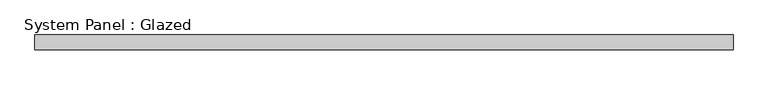
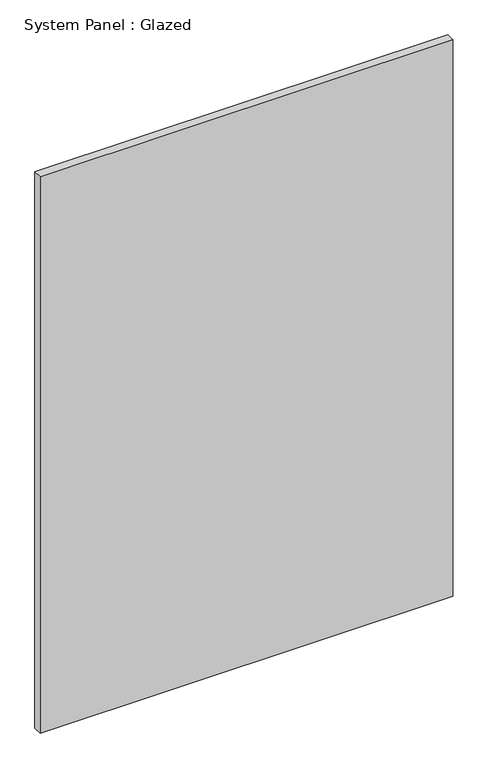
"""IFC4 building model written with IfcOpenShell, lengths in millimetres: plate geometry, System Panel : Glazed."""

from ifc_helpers import new_model, si_unit, origin, origin_with_axes, place, context, project, spatial, polyline, outline, extrude, source, transform, mapped, element, save


def system_panel_glazed_90125d95(model_context):
    return source(origin(), model_context, "Body", "SweptSolid", [
        extrude(outline(polyline([(593.6246112, 19.05), (-593.6246112, 19.05), (-593.6246112, 44.45), (593.6246112, 44.45), (593.6246112, 19.05)])), origin_with_axes(), (0.0, 0.0, 1.0), 1691.9879691),
    ])


if __name__ == "__main__":
    model = new_model("IFC4")
    model_context = context("Model", 3, world=origin())
    ifc_project = project(units=[si_unit("LENGTHUNIT", "METRE", prefix="MILLI")], contexts=[model_context])
    site = spatial("IfcSite", under=ifc_project)
    building = spatial("IfcBuilding", under=site)
    placement = place(None, origin())
    system_panel_glazed_shape = system_panel_glazed_90125d95(model_context)
    element("IfcPlate", 1, ObjectType="System Panel : Glazed", at=placement, inside=building, context=model_context, shape_type="MappedRepresentation", body=[
        mapped(system_panel_glazed_shape, transform((0.0, 0.0, 0.0), x_axis=(1.0, 0.0, 0.0), y_axis=(0.0, 1.0, 0.0), z_axis=(0.0, 0.0, 1.0))),
    ])
    save(model, "model.ifc")

# Revit data of these elements
# Type "System Panel : Glazed"
#   Construction Type Id = "GSP4R"
#   Analytic Construction = "1/8 in Pilkington single glazing"
#   Visual Light Transmittance = 0.9
#   Solar Heat Gain Coefficient = 0.86
#   Heat Transfer Coefficient (U) = 1.18115 BTU/(h·ft²·°F)
#   Define Thermal Properties by = 1
# Element 1 (IfcPlate, "System Panel : Glazed")
#   Materials on its faces: "Glass"
# Materials
#   "Glass": class "Glass", colour RGB 0 128 192, transparency 0.75, Description = "Soda Lime Glass", Cost = 0
